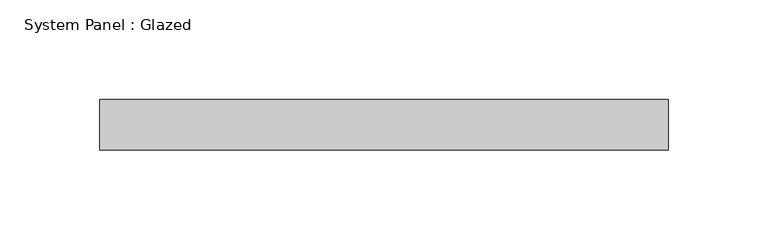
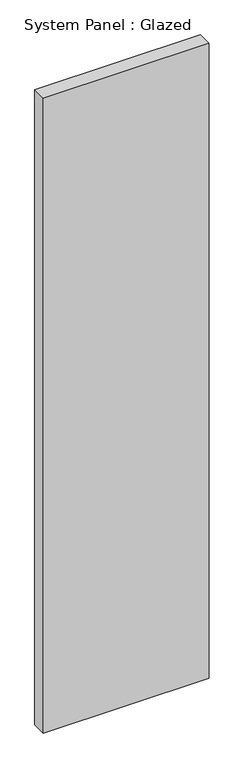
"""IFC4 building model written with IfcOpenShell, lengths in millimetres: plate geometry, System Panel : Glazed."""

from ifc_helpers import new_model, si_unit, origin, origin_with_axes, place, context, project, spatial, polyline, outline, extrude, source, transform, mapped, element, save


def system_panel_glazed_f0550140(model_context):
    return source(origin(), model_context, "Body", "SweptSolid", [
        extrude(outline(polyline([(142.875, 19.05), (-142.875, 19.05), (-142.875, 44.45), (142.875, 44.45), (142.875, 19.05)])), origin_with_axes(), (0.0, 0.0, 1.0), 1155.7),
    ])


if __name__ == "__main__":
    model = new_model("IFC4")
    model_context = context("Model", 3, world=origin())
    ifc_project = project(units=[si_unit("LENGTHUNIT", "METRE", prefix="MILLI")], contexts=[model_context])
    site = spatial("IfcSite", under=ifc_project)
    building = spatial("IfcBuilding", under=site)
    placement = place(None, origin())
    system_panel_glazed_shape = system_panel_glazed_f0550140(model_context)
    element("IfcPlate", 1, ObjectType="System Panel : Glazed", at=placement, inside=building, context=model_context, shape_type="MappedRepresentation", body=[
        mapped(system_panel_glazed_shape, transform((0.0, 0.0, 0.0), x_axis=(1.0, 0.0, 0.0), y_axis=(0.0, 1.0, 0.0), z_axis=(0.0, 0.0, 1.0))),
    ])
    save(model, "model.ifc")

# Revit data of these elements
# Type "System Panel : Glazed"
#   Construction Type Id = "GSP4R"
#   Analytic Construction = "1/8 in Pilkington single glazing"
#   Visual Light Transmittance = 0.9
#   Solar Heat Gain Coefficient = 0.86
#   Heat Transfer Coefficient (U) = 1.18115 BTU/(h·ft²·°F)
#   Define Thermal Properties by = 1
# Element 1 (IfcPlate, "System Panel : Glazed")
#   Materials on its faces: "Glass"
# Materials
#   "Glass": class "Glass", colour RGB 0 128 192, transparency 0.75, Description = "Soda Lime Glass", Cost = 0
